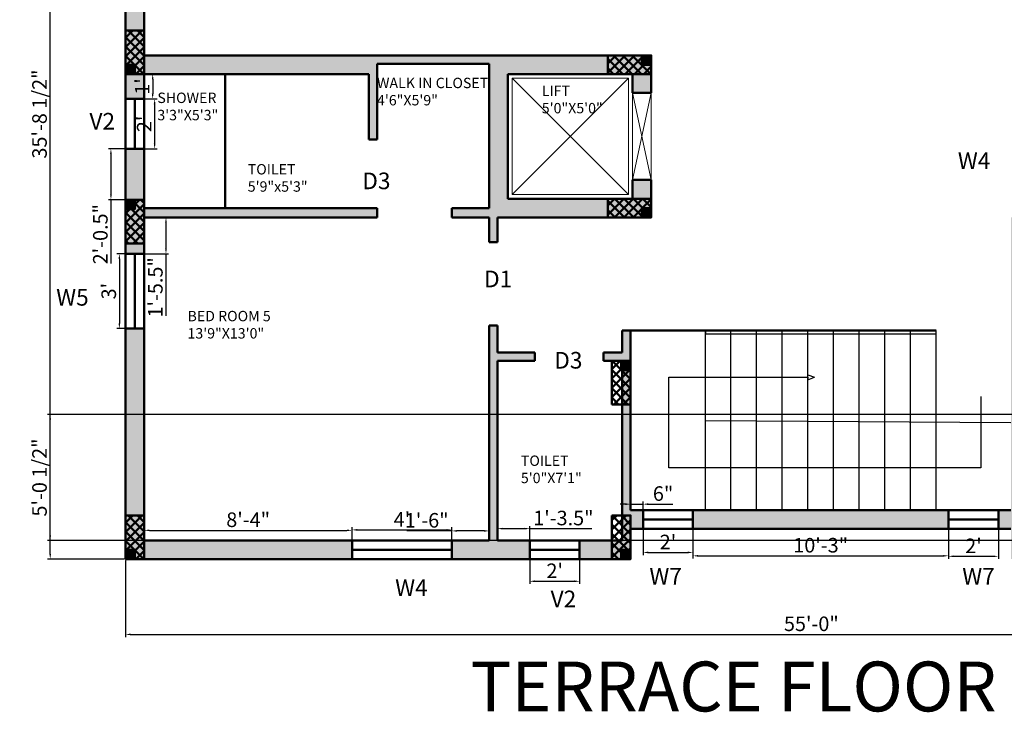
# Model space of a CAD drawing. Units: inches. Extents: x 1749 to 3550, y 1117 to 2383.
# Tile 10 of 15: x 2680 to 3154, y 1169 to 1503. Entities that reach past the tile are written whole.
import ezdxf

# ---------------------------------------------------------------- set-up
doc = ezdxf.new("R2010")
doc.units = ezdxf.units.IN
for name, color, linetype, lineweight in [('A-ANNO-DIMS', 2, 'Continuous', 18), ('A-ANNO-TEXT', 3, 'Continuous', 18), ('A-AREA-IDEN', 7, 'Continuous', 18), ('A-COLS', 10, 'Continuous', 50), ('A-EQPM', 8, 'Continuous', 18), ('A-FLOR-STRS', 53, 'Continuous', 25), ('A-WALL', 7, 'Continuous', 50), ('A-WALL-PATT', 8, 'Continuous', 13)]:
    doc.layers.add(name, color=color, linetype=linetype, lineweight=lineweight)
doc.styles.get("Standard").update_dxf_attribs({"font": 'arial.ttf'})
doc.dimstyles.new('ISO-25', dxfattribs={"dimtxt": 7, "dimasz": 2.5, "dimexe": 1.25, "dimexo": 0.625, "dimtad": 1, "dimdec": 1, "dimlunit": 3, "dimtxsty": 'Standard', "dimcen": 2.5, "dimadec": 0, "dimazin": 0, "dimtfac": 1, "dimtdec": 1, "dimtmove": 0, "dimatfit": 3, "dimfxl": 1, "dimarcsym": 0})

# ---------------------------------------------------------------- blocks, each defined once
blk = doc.blocks.new('*D107')
at = {"layer": 'A-ANNO-DIMS', "color": 0, "lineweight": -2, "ltscale": 0.5, "transparency": 16777216}
for p, q in [((2740.46, 1476.39), (2745.15, 1476.39)), ((2743.9, 1473.89), (2743.9, 1466.89)), ((2740.46, 1464.39), (2745.15, 1464.39))]:
    blk.add_line(p, q, dxfattribs=at)
at = {"layer": 'A-ANNO-DIMS', "color": 0, "ltscale": 0.5, "transparency": 16777216}
for points in [[(2743.48, 1473.89), (2744.31, 1473.89), (2743.9, 1476.39)], [(2743.48, 1466.89), (2744.31, 1466.89), (2743.9, 1464.39)]]:
    blk.add_solid(points, dxfattribs=at)
at = {"layer": 'Defpoints', "color": 0, "ltscale": 0.5, "transparency": 16777216}
for p in [(2739.84, 1476.39), (2739.84, 1464.39), (2743.9, 1464.39)]:
    blk.add_point(p, dxfattribs=at)
at = {"layer": 'A-ANNO-DIMS', "color": 0, "ltscale": 0.5, "transparency": 16777216, "insert": (2739.76, 1470.39), "char_height": 7, "attachment_point": 5, "rotation": 90}
blk.add_mtext("1'", dxfattribs=at)
blk = doc.blocks.new('*D108')
at = {"layer": 'A-ANNO-DIMS', "color": 0, "lineweight": -2, "ltscale": 0.5, "transparency": 16777216}
for p, q in [((2740.46, 1464.39), (2746.09, 1464.39)), ((2744.84, 1461.89), (2744.84, 1442.89)), ((2740.46, 1440.39), (2746.09, 1440.39))]:
    blk.add_line(p, q, dxfattribs=at)
at = {"layer": 'A-ANNO-DIMS', "color": 0, "ltscale": 0.5, "transparency": 16777216}
for points in [[(2744.42, 1461.89), (2745.25, 1461.89), (2744.84, 1464.39)], [(2744.42, 1442.89), (2745.25, 1442.89), (2744.84, 1440.39)]]:
    blk.add_solid(points, dxfattribs=at)
at = {"layer": 'Defpoints', "color": 0, "ltscale": 0.5, "transparency": 16777216}
for p in [(2739.84, 1464.39), (2739.84, 1440.39), (2744.84, 1440.39)]:
    blk.add_point(p, dxfattribs=at)
at = {"layer": 'A-ANNO-DIMS', "color": 0, "ltscale": 0.5, "transparency": 16777216, "insert": (2740.7, 1452.39), "char_height": 7, "attachment_point": 5, "rotation": 90}
blk.add_mtext("2'", dxfattribs=at)
blk = doc.blocks.new('*D109')
at = {"layer": 'A-ANNO-DIMS', "color": 0, "lineweight": -2, "ltscale": 0.5, "transparency": 16777216}
for p, q in [((2730.21, 1440.39), (2722.56, 1440.39)), ((2723.81, 1437.89), (2723.81, 1418.37)), ((2730.21, 1415.87), (2722.56, 1415.87)), ((2723.81, 1415.87), (2723.81, 1385.23))]:
    blk.add_line(p, q, dxfattribs=at)
at = {"layer": 'A-ANNO-DIMS', "color": 0, "ltscale": 0.5, "transparency": 16777216}
for points in [[(2723.39, 1437.89), (2724.22, 1437.89), (2723.81, 1440.39)], [(2723.39, 1418.37), (2724.22, 1418.37), (2723.81, 1415.87)]]:
    blk.add_solid(points, dxfattribs=at)
at = {"layer": 'Defpoints', "color": 0, "ltscale": 0.5, "transparency": 16777216}
for p in [(2730.84, 1440.39), (2723.81, 1415.87), (2730.84, 1415.87)]:
    blk.add_point(p, dxfattribs=at)
at = {"layer": 'A-ANNO-DIMS', "color": 0, "ltscale": 0.5, "transparency": 16777216, "insert": (2719.61, 1399.3), "char_height": 7, "attachment_point": 5, "rotation": 90}
blk.add_mtext('2\'-0.5"', dxfattribs=at)
blk = doc.blocks.new('*D110')
at = {"layer": 'A-ANNO-DIMS', "color": 0, "lineweight": -2, "ltscale": 0.5, "transparency": 16777216}
for p, q in [((2740.46, 1407.39), (2751.54, 1407.39)), ((2750.29, 1404.89), (2750.29, 1392.39)), ((2740.46, 1389.89), (2751.54, 1389.89)), ((2750.29, 1389.89), (2750.29, 1360.03))]:
    blk.add_line(p, q, dxfattribs=at)
at = {"layer": 'A-ANNO-DIMS', "color": 0, "ltscale": 0.5, "transparency": 16777216}
for points in [[(2749.87, 1404.89), (2750.71, 1404.89), (2750.29, 1407.39)], [(2749.87, 1392.39), (2750.71, 1392.39), (2750.29, 1389.89)]]:
    blk.add_solid(points, dxfattribs=at)
at = {"layer": 'Defpoints', "color": 0, "ltscale": 0.5, "transparency": 16777216}
for p in [(2739.84, 1407.39), (2739.84, 1389.89), (2750.29, 1389.89)]:
    blk.add_point(p, dxfattribs=at)
at = {"layer": 'A-ANNO-DIMS', "color": 0, "ltscale": 0.5, "transparency": 16777216, "insert": (2746.09, 1373.71), "char_height": 7, "attachment_point": 5, "rotation": 90}
blk.add_mtext('1\'-5.5"', dxfattribs=at)
blk = doc.blocks.new('*D111')
at = {"layer": 'A-ANNO-DIMS', "color": 0, "lineweight": -2, "ltscale": 0.5, "transparency": 16777216}
for p, q in [((2730.21, 1389.89), (2726.61, 1389.89)), ((2727.86, 1387.39), (2727.86, 1356.39)), ((2730.21, 1353.89), (2726.61, 1353.89))]:
    blk.add_line(p, q, dxfattribs=at)
at = {"layer": 'A-ANNO-DIMS', "color": 0, "ltscale": 0.5, "transparency": 16777216}
for points in [[(2727.45, 1387.39), (2728.28, 1387.39), (2727.86, 1389.89)], [(2727.45, 1356.39), (2728.28, 1356.39), (2727.86, 1353.89)]]:
    blk.add_solid(points, dxfattribs=at)
at = {"layer": 'Defpoints', "color": 0, "ltscale": 0.5, "transparency": 16777216}
for p in [(2730.84, 1389.89), (2727.86, 1353.89), (2730.84, 1353.89)]:
    blk.add_point(p, dxfattribs=at)
at = {"layer": 'A-ANNO-DIMS', "color": 0, "ltscale": 0.5, "transparency": 16777216, "insert": (2723.66, 1371.89), "char_height": 7, "attachment_point": 5, "rotation": 90}
blk.add_mtext("3'", dxfattribs=at)
blk = doc.blocks.new('*D112')
at = {"layer": 'A-ANNO-DIMS', "color": 0, "lineweight": -2, "ltscale": 0.5, "transparency": 16777216}
for p, q in [((2739.84, 1252.51), (2739.84, 1257.99)), ((2742.34, 1256.74), (2837.34, 1256.74)), ((2839.84, 1252.51), (2839.84, 1257.99))]:
    blk.add_line(p, q, dxfattribs=at)
at = {"layer": 'A-ANNO-DIMS', "color": 0, "ltscale": 0.5, "transparency": 16777216}
for points in [[(2742.34, 1257.15), (2742.34, 1256.32), (2739.84, 1256.74)], [(2837.34, 1257.15), (2837.34, 1256.32), (2839.84, 1256.74)]]:
    blk.add_solid(points, dxfattribs=at)
at = {"layer": 'Defpoints', "color": 0, "ltscale": 0.5, "transparency": 16777216}
for p in [(2839.84, 1256.74), (2739.84, 1251.89), (2839.84, 1251.89)]:
    blk.add_point(p, dxfattribs=at)
at = {"layer": 'A-ANNO-DIMS', "color": 0, "ltscale": 0.5, "transparency": 16777216, "insert": (2789.84, 1260.93), "char_height": 7, "attachment_point": 5}
blk.add_mtext('8\'-4"', dxfattribs=at)
blk = doc.blocks.new('*D113')
at = {"layer": 'A-ANNO-DIMS', "color": 0, "lineweight": -2, "ltscale": 0.5, "transparency": 16777216}
for p, q in [((2839.84, 1252.51), (2839.84, 1258.21)), ((2842.34, 1256.96), (2885.34, 1256.96)), ((2887.84, 1252.51), (2887.84, 1258.21))]:
    blk.add_line(p, q, dxfattribs=at)
at = {"layer": 'A-ANNO-DIMS', "color": 0, "ltscale": 0.5, "transparency": 16777216}
for points in [[(2842.34, 1257.37), (2842.34, 1256.54), (2839.84, 1256.96)], [(2885.34, 1257.37), (2885.34, 1256.54), (2887.84, 1256.96)]]:
    blk.add_solid(points, dxfattribs=at)
at = {"layer": 'Defpoints', "color": 0, "ltscale": 0.5, "transparency": 16777216}
for p in [(2887.84, 1256.96), (2839.84, 1251.89), (2887.84, 1251.89)]:
    blk.add_point(p, dxfattribs=at)
at = {"layer": 'A-ANNO-DIMS', "color": 0, "ltscale": 0.5, "transparency": 16777216, "insert": (2863.84, 1261.08), "char_height": 7, "attachment_point": 5}
blk.add_mtext("4'", dxfattribs=at)
blk = doc.blocks.new('*D114')
at = {"layer": 'A-ANNO-DIMS', "color": 0, "lineweight": -2, "ltscale": 0.5, "transparency": 16777216}
for p, q in [((2887.84, 1256.46), (2866.14, 1256.46)), ((2887.84, 1252.51), (2887.84, 1257.71)), ((2903.34, 1256.46), (2890.34, 1256.46)), ((2905.84, 1252.51), (2905.84, 1257.71))]:
    blk.add_line(p, q, dxfattribs=at)
at = {"layer": 'A-ANNO-DIMS', "color": 0, "ltscale": 0.5, "transparency": 16777216}
for points in [[(2890.34, 1256.88), (2890.34, 1256.05), (2887.84, 1256.46)], [(2903.34, 1256.88), (2903.34, 1256.05), (2905.84, 1256.46)]]:
    blk.add_solid(points, dxfattribs=at)
at = {"layer": 'Defpoints', "color": 0, "ltscale": 0.5, "transparency": 16777216}
for p in [(2887.84, 1256.46), (2887.84, 1251.89), (2905.84, 1251.89)]:
    blk.add_point(p, dxfattribs=at)
at = {"layer": 'A-ANNO-DIMS', "color": 0, "ltscale": 0.5, "transparency": 16777216, "insert": (2875.74, 1260.66), "char_height": 7, "attachment_point": 5}
blk.add_mtext('1\'-6"', dxfattribs=at)
blk = doc.blocks.new('*D115')
at = {"layer": 'A-ANNO-DIMS', "color": 0, "lineweight": -2, "ltscale": 0.5, "transparency": 16777216}
for p, q in [((2909.84, 1252.51), (2909.84, 1258.81)), ((2912.34, 1257.56), (2922.84, 1257.56)), ((2925.34, 1252.51), (2925.34, 1258.81)), ((2925.34, 1257.56), (2955.19, 1257.56))]:
    blk.add_line(p, q, dxfattribs=at)
at = {"layer": 'A-ANNO-DIMS', "color": 0, "ltscale": 0.5, "transparency": 16777216}
for points in [[(2912.34, 1257.98), (2912.34, 1257.14), (2909.84, 1257.56)], [(2922.84, 1257.98), (2922.84, 1257.14), (2925.34, 1257.56)]]:
    blk.add_solid(points, dxfattribs=at)
at = {"layer": 'Defpoints', "color": 0, "ltscale": 0.5, "transparency": 16777216}
for p in [(2925.34, 1257.56), (2909.84, 1251.89), (2925.34, 1251.89)]:
    blk.add_point(p, dxfattribs=at)
at = {"layer": 'A-ANNO-DIMS', "color": 0, "ltscale": 0.5, "transparency": 16777216, "insert": (2941.51, 1261.76), "char_height": 7, "attachment_point": 5}
blk.add_mtext('1\'-3.5"', dxfattribs=at)
blk = doc.blocks.new('*D116')
at = {"layer": 'A-ANNO-DIMS', "color": 0, "lineweight": -2, "ltscale": 0.5, "transparency": 16777216}
for p, q in [((2925.34, 1242.26), (2925.34, 1230.97)), ((2949.34, 1242.26), (2949.34, 1230.97)), ((2927.84, 1232.22), (2946.84, 1232.22))]:
    blk.add_line(p, q, dxfattribs=at)
at = {"layer": 'A-ANNO-DIMS', "color": 0, "ltscale": 0.5, "transparency": 16777216}
for points in [[(2927.84, 1232.63), (2927.84, 1231.8), (2925.34, 1232.22)], [(2946.84, 1232.63), (2946.84, 1231.8), (2949.34, 1232.22)]]:
    blk.add_solid(points, dxfattribs=at)
at = {"layer": 'Defpoints', "color": 0, "ltscale": 0.5, "transparency": 16777216}
for p in [(2925.34, 1242.89), (2949.34, 1242.89), (2949.34, 1232.22)]:
    blk.add_point(p, dxfattribs=at)
at = {"layer": 'A-ANNO-DIMS', "color": 0, "ltscale": 0.5, "transparency": 16777216, "insert": (2937.34, 1236.36), "char_height": 7, "attachment_point": 5}
blk.add_mtext("2'", dxfattribs=at)
blk = doc.blocks.new('*D117')
at = {"layer": 'A-ANNO-DIMS', "color": 0, "lineweight": -2, "ltscale": 0.5, "transparency": 16777216}
for p, q in [((2973.84, 1267.01), (2973.84, 1270.59)), ((2979.84, 1267.01), (2979.84, 1270.59)), ((2971.34, 1269.34), (2968.84, 1269.34)), ((2973.84, 1269.34), (2979.84, 1269.34)), ((2982.34, 1269.34), (2994.17, 1269.34))]:
    blk.add_line(p, q, dxfattribs=at)
at = {"layer": 'A-ANNO-DIMS', "color": 0, "ltscale": 0.5, "transparency": 16777216}
for points in [[(2971.34, 1269.76), (2971.34, 1268.92), (2973.84, 1269.34)], [(2982.34, 1269.76), (2982.34, 1268.92), (2979.84, 1269.34)]]:
    blk.add_solid(points, dxfattribs=at)
at = {"layer": 'Defpoints', "color": 0, "ltscale": 0.5, "transparency": 16777216}
for p in [(2973.84, 1266.39), (2979.84, 1269.34), (2979.84, 1266.39)]:
    blk.add_point(p, dxfattribs=at)
at = {"layer": 'A-ANNO-DIMS', "color": 0, "ltscale": 0.5, "transparency": 16777216, "insert": (2989.5, 1273.54), "char_height": 7, "attachment_point": 5}
blk.add_mtext('6"', dxfattribs=at)
blk = doc.blocks.new('*D118')
at = {"layer": 'A-ANNO-DIMS', "color": 0, "lineweight": -2, "ltscale": 0.5, "transparency": 16777216}
for p, q in [((2979.84, 1256.76), (2979.84, 1244.85)), ((3003.84, 1256.76), (3003.84, 1244.85)), ((2982.34, 1246.1), (3001.34, 1246.1))]:
    blk.add_line(p, q, dxfattribs=at)
at = {"layer": 'A-ANNO-DIMS', "color": 0, "ltscale": 0.5, "transparency": 16777216}
for points in [[(2982.34, 1246.51), (2982.34, 1245.68), (2979.84, 1246.1)], [(3001.34, 1246.51), (3001.34, 1245.68), (3003.84, 1246.1)]]:
    blk.add_solid(points, dxfattribs=at)
at = {"layer": 'Defpoints', "color": 0, "ltscale": 0.5, "transparency": 16777216}
for p in [(2979.84, 1257.39), (3003.84, 1257.39), (3003.84, 1246.1)]:
    blk.add_point(p, dxfattribs=at)
at = {"layer": 'A-ANNO-DIMS', "color": 0, "ltscale": 0.5, "transparency": 16777216, "insert": (2991.84, 1250.23), "char_height": 7, "attachment_point": 5}
blk.add_mtext("2'", dxfattribs=at)
blk = doc.blocks.new('*D119')
at = {"layer": 'A-ANNO-DIMS', "color": 0, "lineweight": -2, "ltscale": 0.5, "transparency": 16777216}
for p, q in [((3003.84, 1256.76), (3003.84, 1243.22)), ((3126.84, 1256.76), (3126.84, 1243.22)), ((3006.34, 1244.47), (3124.34, 1244.47))]:
    blk.add_line(p, q, dxfattribs=at)
at = {"layer": 'A-ANNO-DIMS', "color": 0, "ltscale": 0.5, "transparency": 16777216}
for points in [[(3006.34, 1244.88), (3006.34, 1244.05), (3003.84, 1244.47)], [(3124.34, 1244.88), (3124.34, 1244.05), (3126.84, 1244.47)]]:
    blk.add_solid(points, dxfattribs=at)
at = {"layer": 'Defpoints', "color": 0, "ltscale": 0.5, "transparency": 16777216}
for p in [(3003.84, 1257.39), (3126.84, 1257.39), (3126.84, 1244.47)]:
    blk.add_point(p, dxfattribs=at)
at = {"layer": 'A-ANNO-DIMS', "color": 0, "ltscale": 0.5, "transparency": 16777216, "insert": (3065.34, 1248.67), "char_height": 7, "attachment_point": 5}
blk.add_mtext('10\'-3"', dxfattribs=at)
blk = doc.blocks.new('*D120')
at = {"layer": 'A-ANNO-DIMS', "color": 0, "lineweight": -2, "ltscale": 0.5, "transparency": 16777216}
for p, q in [((3126.84, 1256.76), (3126.84, 1242.98)), ((3150.84, 1256.76), (3150.84, 1242.98)), ((3129.34, 1244.23), (3148.34, 1244.23))]:
    blk.add_line(p, q, dxfattribs=at)
at = {"layer": 'A-ANNO-DIMS', "color": 0, "ltscale": 0.5, "transparency": 16777216}
for points in [[(3129.34, 1244.65), (3129.34, 1243.82), (3126.84, 1244.23)], [(3148.34, 1244.65), (3148.34, 1243.82), (3150.84, 1244.23)]]:
    blk.add_solid(points, dxfattribs=at)
at = {"layer": 'Defpoints', "color": 0, "ltscale": 0.5, "transparency": 16777216}
for p in [(3126.84, 1257.39), (3150.84, 1257.39), (3150.84, 1244.23)]:
    blk.add_point(p, dxfattribs=at)
at = {"layer": 'A-ANNO-DIMS', "color": 0, "ltscale": 0.5, "transparency": 16777216, "insert": (3138.84, 1248.37), "char_height": 7, "attachment_point": 5}
blk.add_mtext("2'", dxfattribs=at)
blk = doc.blocks.new('LIFT-A')
at = {"ltscale": 0.2}
for p, q in [((0, 56), (56, 56)), ((0, 56), (0, 0)), ((56, 56), (0, 0)), ((0, 56), (56, 0)), ((56, 56), (56, 0)), ((0, 0), (56, 0))]:
    blk.add_line(p, q, dxfattribs=at)
blk = doc.blocks.new('*D199')
at = {"layer": 'A-ANNO-DIMS', "color": 0, "lineweight": -2, "ltscale": 0.5, "transparency": 16777216}
for p, q in [((2730.84, 1242.26), (2730.84, 1205.39)), ((3390.84, 1242.26), (3390.84, 1205.39)), ((2733.34, 1206.64), (3388.34, 1206.64))]:
    blk.add_line(p, q, dxfattribs=at)
at = {"layer": 'A-ANNO-DIMS', "color": 0, "ltscale": 0.5, "transparency": 16777216}
for points in [[(2733.34, 1207.05), (2733.34, 1206.22), (2730.84, 1206.64)], [(3388.34, 1207.05), (3388.34, 1206.22), (3390.84, 1206.64)]]:
    blk.add_solid(points, dxfattribs=at)
at = {"layer": 'Defpoints', "color": 0, "ltscale": 0.5, "transparency": 16777216}
for p in [(2730.84, 1242.89), (3390.84, 1242.89), (3390.84, 1206.64)]:
    blk.add_point(p, dxfattribs=at)
at = {"layer": 'A-ANNO-DIMS', "color": 0, "ltscale": 0.5, "transparency": 16777216, "insert": (3060.84, 1210.84), "char_height": 7, "attachment_point": 5}
blk.add_mtext('55\'-0"', dxfattribs=at)
blk = doc.blocks.new('*D200')
at = {"layer": 'A-ANNO-DIMS', "color": 0, "lineweight": -2, "ltscale": 0.5, "transparency": 16777216}
for p, q in [((2730.21, 1671.39), (2693.34, 1671.39)), ((2694.59, 1245.39), (2694.59, 1668.89)), ((2730.21, 1242.89), (2693.34, 1242.89))]:
    blk.add_line(p, q, dxfattribs=at)
at = {"layer": 'A-ANNO-DIMS', "color": 0, "ltscale": 0.5, "transparency": 16777216}
for points in [[(2694.17, 1668.89), (2695, 1668.89), (2694.59, 1671.39)], [(2694.17, 1245.39), (2695, 1245.39), (2694.59, 1242.89)]]:
    blk.add_solid(points, dxfattribs=at)
at = {"layer": 'Defpoints', "color": 0, "ltscale": 0.5, "transparency": 16777216}
for p in [(2694.59, 1671.39), (2730.84, 1671.39), (2730.84, 1242.89)]:
    blk.add_point(p, dxfattribs=at)
at = {"layer": 'A-ANNO-DIMS', "color": 0, "ltscale": 0.5, "transparency": 16777216, "insert": (2690.34, 1457.14), "char_height": 7, "attachment_point": 5, "rotation": 90}
blk.add_mtext('35\'-8 1/2"', dxfattribs=at)
blk = doc.blocks.new('*D204')
at = {"layer": 'A-ANNO-DIMS', "color": 0, "lineweight": -2, "ltscale": 0.5, "transparency": 16777216}
for p, q in [((3202.94, 1312.45), (2693.34, 1312.45)), ((2694.59, 1254.39), (2694.59, 1309.95)), ((3165.21, 1251.89), (2693.34, 1251.89))]:
    blk.add_line(p, q, dxfattribs=at)
at = {"layer": 'A-ANNO-DIMS', "color": 0, "ltscale": 0.5, "transparency": 16777216}
for points in [[(2694.17, 1309.95), (2695, 1309.95), (2694.59, 1312.45)], [(2694.17, 1254.39), (2695, 1254.39), (2694.59, 1251.89)]]:
    blk.add_solid(points, dxfattribs=at)
at = {"layer": 'Defpoints', "color": 0, "ltscale": 0.5, "transparency": 16777216}
for p in [(2694.59, 1312.45), (3203.57, 1312.45), (3165.84, 1251.89)]:
    blk.add_point(p, dxfattribs=at)
at = {"layer": 'A-ANNO-DIMS', "color": 0, "ltscale": 0.5, "transparency": 16777216, "insert": (2690.34, 1282.17), "char_height": 7, "attachment_point": 5, "rotation": 90}
blk.add_mtext('5\'-0 1/2"', dxfattribs=at)

msp = doc.modelspace()

# ---------------------------------------------------------------- hatches: boundary and pattern name
at = {"layer": 'A-COLS', "ltscale": 10}
h = msp.add_hatch(dxfattribs=at)
h.set_pattern_fill('ANSI37', color=256, angle=270)
h.set_pattern_definition([(315, (1372.7294, 3148.631), (2.245064, 2.245064), []), (45, (1372.7294, 3148.631), (-2.245064, 2.245064), [])])
h.paths.add_polyline_path([(2730.84, 1476.39), (2739.84, 1476.39), (2739.84, 1497.39), (2730.84, 1497.39)])
h = msp.add_hatch(dxfattribs=at)
h.set_pattern_fill('ANSI37', color=256, angle=360)
h.set_pattern_definition([(45, (1311.591, 90.5872), (-2.245064, 2.245064), []), (135, (1311.591, 90.5872), (-2.245064, -2.245064), [])])
h.paths.add_polyline_path([(2962.84, 1485.39), (2962.84, 1476.39), (2983.84, 1476.39), (2983.84, 1485.39)])
h = msp.add_hatch(color=256, dxfattribs=at)
h.dxf.hatch_style = 1
h.paths.add_polyline_path([(2983.84, 1485.39), (2979.34, 1485.39), (2979.34, 1480.89), (2983.84, 1480.89)])
h = msp.add_hatch(color=256, dxfattribs=at)
h.dxf.hatch_style = 1
h.paths.add_polyline_path([(2735.34, 1476.39), (2735.34, 1480.89), (2730.84, 1480.89), (2730.84, 1476.39)])
h = msp.add_hatch(color=256, dxfattribs=at)
h.dxf.hatch_style = 1
h.paths.add_polyline_path([(2730.84, 1415.87), (2730.84, 1411.37), (2735.34, 1411.37), (2735.34, 1415.87)])
h = msp.add_hatch(dxfattribs=at)
h.set_pattern_fill('ANSI37', color=256, angle=90)
h.set_pattern_definition([(135, (4078.1257, -256.377), (-2.245064, -2.245064), []), (225, (4078.1257, -256.377), (2.245064, -2.245064), [])])
h.paths.add_polyline_path([(2730.84, 1394.87), (2739.84, 1394.87), (2739.84, 1415.87), (2730.84, 1415.87)])
h = msp.add_hatch(dxfattribs=at)
h.set_pattern_fill('ANSI37', color=256, angle=360)
h.set_pattern_definition([(45, (1311.591, 49.2816), (-2.245064, 2.245064), []), (135, (1311.591, 49.2816), (-2.245064, -2.245064), [])])
h.paths.add_polyline_path([(2983.84, 1407.39), (2983.84, 1416.39), (2962.84, 1416.39), (2962.84, 1407.39)])
h = msp.add_hatch(color=256, dxfattribs=at)
h.dxf.hatch_style = 1
h.paths.add_polyline_path([(2983.84, 1411.89), (2979.34, 1411.89), (2979.34, 1407.39), (2983.84, 1407.39)])
h = msp.add_hatch(dxfattribs=at)
h.set_pattern_fill('ANSI37', color=256, angle=90)
h.set_pattern_definition([(135, (4331.9415, -333.8625), (-2.245064, -2.245064), []), (225, (4331.9415, -333.8625), (2.245064, -2.245064), [])])
h.paths.add_polyline_path([(2973.84, 1338.38), (2964.84, 1338.38), (2964.84, 1317.38), (2973.84, 1317.38)])
h = msp.add_hatch(color=256, dxfattribs=at)
h.dxf.hatch_style = 1
h.paths.add_polyline_path([(2969.34, 1338.38), (2969.34, 1333.88), (2973.84, 1333.88), (2973.84, 1338.38)])
h = msp.add_hatch(dxfattribs=at)
h.set_pattern_fill('ANSI37', color=256, angle=270)
h.set_pattern_definition([(315, (1372.7294, 2915.132), (2.245064, 2.245064), []), (45, (1372.7294, 2915.132), (-2.245064, 2.245064), [])])
h.paths.add_polyline_path([(2730.84, 1242.89), (2739.84, 1242.89), (2739.84, 1263.89), (2730.84, 1263.89)])
h = msp.add_hatch(dxfattribs=at)
h.set_pattern_fill('ANSI37', color=256, angle=270)
h.set_pattern_definition([(315, (1583.087, 2915.132), (2.245064, 2.245064), []), (45, (1583.087, 2915.132), (-2.245064, 2.245064), [])])
h.paths.add_polyline_path([(2973.84, 1263.89), (2964.84, 1263.89), (2964.84, 1242.89), (2973.84, 1242.89)])
h = msp.add_hatch(color=256, dxfattribs=at)
h.dxf.hatch_style = 1
h.paths.add_polyline_path([(2735.34, 1242.89), (2735.34, 1247.39), (2730.84, 1247.39), (2730.84, 1242.89)])
h = msp.add_hatch(color=256, dxfattribs=at)
h.dxf.hatch_style = 1
h.paths.add_polyline_path([(2973.84, 1242.89), (2973.84, 1247.39), (2969.34, 1247.39), (2969.34, 1242.89)])
at = {"layer": 'A-WALL-PATT', "ltscale": 0.5}
h = msp.add_hatch(color=256, dxfattribs=at)
h.dxf.hatch_style = 1
h.paths.add_polyline_path([(2798.34, 1662.39), (2798.34, 1671.39), (2730.84, 1671.39), (2730.84, 1464.39), (2739.84, 1464.39), (2739.84, 1476.39), (2847.84, 1476.39), (2847.84, 1444.89), (2851.84, 1444.89), (2851.84, 1481.39), (2905.84, 1481.39), (2905.84, 1411.89), (2887.84, 1411.89), (2887.84, 1407.39), (2905.84, 1407.39), (2905.84, 1395.39), (2909.84, 1395.39), (2909.84, 1407.39), (2973.84, 1407.39), (2983.84, 1407.39), (2983.84, 1425.39), (2974.84, 1425.39), (2974.84, 1416.39), (2914.84, 1416.39), (2914.84, 1476.39), (2974.84, 1476.39), (2974.84, 1467.39), (2983.84, 1467.39), (2983.84, 1476.39), (2983.84, 1485.39), (2739.84, 1485.39), (2739.84, 1662.39)])
h = msp.add_hatch(color=256, dxfattribs=at)
h.dxf.hatch_style = 1
h.paths.add_polyline_path([(2739.84, 1407.39), (2851.84, 1407.39), (2851.84, 1411.89), (2847.84, 1411.89), (2739.84, 1411.89), (2739.84, 1440.39), (2730.84, 1440.39), (2730.84, 1389.89), (2739.84, 1389.89)])
h = msp.add_hatch(color=256, dxfattribs=at)
h.dxf.hatch_style = 1
h.paths.add_polyline_path([(3156.84, 1266.39), (3150.84, 1266.39), (3150.84, 1257.39), (3156.84, 1257.39), (3156.84, 1242.89), (3165.84, 1242.89), (3165.84, 1251.89), (3165.84, 1407.39), (3156.84, 1407.39)])
h = msp.add_hatch(color=256, dxfattribs=at)
h.dxf.hatch_style = 1
h.paths.add_polyline_path([(2905.84, 1251.89), (2887.84, 1251.89), (2887.84, 1242.89), (2925.34, 1242.89), (2925.34, 1251.89), (2909.84, 1251.89), (2909.84, 1338.39), (2927.84, 1338.39), (2927.84, 1342.39), (2909.84, 1342.39), (2909.84, 1355.39), (2905.84, 1355.39)])
h = msp.add_hatch(color=256, dxfattribs=at)
h.dxf.hatch_style = 1
h.paths.add_polyline_path([(2739.84, 1353.89), (2730.84, 1353.89), (2730.84, 1242.89), (2839.84, 1242.89), (2839.84, 1251.89), (2739.84, 1251.89)])
h = msp.add_hatch(color=256, dxfattribs=at)
h.dxf.hatch_style = 1
h.paths.add_polyline_path([(2973.84, 1242.89), (2973.84, 1257.39), (2979.84, 1257.39), (2979.84, 1266.39), (2973.84, 1266.39), (2973.84, 1352.89), (2969.84, 1352.89), (2969.84, 1342.39), (2960.84, 1342.39), (2960.84, 1338.39), (2969.84, 1338.39), (2969.84, 1251.89), (2949.34, 1251.89), (2949.34, 1242.89)])
h = msp.add_hatch(color=256, dxfattribs=at)
h.dxf.hatch_style = 1
h.paths.add_polyline_path([(3126.84, 1257.39), (3126.84, 1266.39), (3003.84, 1266.39), (3003.84, 1257.39)])

# ---------------------------------------------------------------- linework, layer by layer
at = {"layer": 'A-COLS', "ltscale": 10}
for points in [[(2739.84, 1497.39), (2739.84, 1476.39), (2730.84, 1476.39), (2730.84, 1497.39)], [(2962.84, 1476.39), (2983.84, 1476.39), (2983.84, 1485.39), (2962.84, 1485.39)], [(2983.84, 1480.89), (2983.84, 1485.39), (2979.34, 1485.39), (2979.34, 1480.89)], [(2735.34, 1476.39), (2730.84, 1476.39), (2730.84, 1480.89), (2735.34, 1480.89)], [(2735.34, 1415.87), (2730.84, 1415.87), (2730.84, 1411.37), (2735.34, 1411.37)], [(2739.84, 1394.87), (2739.84, 1415.87), (2730.84, 1415.87), (2730.84, 1394.87)], [(2962.84, 1416.39), (2983.84, 1416.39), (2983.84, 1407.39), (2962.84, 1407.39)], [(2983.84, 1411.89), (2983.84, 1407.39), (2979.34, 1407.39), (2979.34, 1411.89)], [(2964.84, 1317.38), (2964.84, 1338.38), (2973.84, 1338.38), (2973.84, 1317.38)], [(2969.34, 1338.38), (2973.84, 1338.38), (2973.84, 1333.88), (2969.34, 1333.88)], [(2739.84, 1263.89), (2739.84, 1242.89), (2730.84, 1242.89), (2730.84, 1263.89)], [(2964.84, 1263.89), (2964.84, 1242.89), (2973.84, 1242.89), (2973.84, 1263.89)], [(2735.34, 1242.89), (2730.84, 1242.89), (2730.84, 1247.39), (2735.34, 1247.39)], [(2969.34, 1242.89), (2973.84, 1242.89), (2973.84, 1247.39), (2969.34, 1247.39)]]:
    msp.add_lwpolyline(points, close=True, dxfattribs=at)
at = {"layer": 'A-EQPM', "ltscale": 0.5}
for p, q in [((2914.84, 1476.39), (2914.84, 1474.39)), ((2974.84, 1467.39), (2974.84, 1425.39)), ((2983.84, 1467.39), (2974.84, 1467.39)), ((2974.84, 1467.39), (2983.84, 1425.39)), ((2974.84, 1425.39), (2983.84, 1467.39)), ((2983.84, 1425.39), (2983.84, 1467.39)), ((2974.84, 1425.39), (2983.84, 1425.39)), ((2983.84, 1425.39), (2974.84, 1425.39))]:
    msp.add_line(p, q, dxfattribs=at)
at = {"layer": 'A-FLOR-STRS', "ltscale": 0.5}
for p, q in [((3009.84, 1266.39), (3009.84, 1352.89)), ((3009.84, 1352.89), (3009.84, 1351.39)), ((3009.84, 1351.39), (3120.84, 1351.39)), ((3022.17, 1266.39), (3022.17, 1352.89)), ((3034.5, 1266.39), (3034.5, 1352.89)), ((3046.84, 1266.39), (3046.84, 1352.89)), ((3059.17, 1266.39), (3059.17, 1352.89)), ((3071.5, 1266.39), (3071.5, 1352.89)), ((3083.84, 1266.39), (3083.84, 1352.89)), ((3096.17, 1266.39), (3096.17, 1352.89)), ((3108.5, 1266.39), (3108.5, 1352.89)), ((3120.84, 1266.39), (3120.84, 1352.89)), ((3120.84, 1266.39), (3120.84, 1351.39)), ((3059.17, 1330.41), (3059.17, 1331.66)), ((3059.17, 1331.66), (3062.37, 1330.41)), ((2992.28, 1286.82), (2992.28, 1330.41)), ((2992.28, 1330.41), (3059.17, 1330.41)), ((3059.17, 1330.41), (3059.17, 1329.16)), ((3059.17, 1329.16), (3062.37, 1330.41)), ((3142.39, 1321.15), (3142.39, 1286.82)), ((3009.84, 1309.64), (3156.84, 1308.64)), ((3142.39, 1286.82), (2992.28, 1286.82))]:
    msp.add_line(p, q, dxfattribs=at)
at = {"layer": 'A-WALL', "ltscale": 0.5}
for p, q in [((2730.84, 1671.39), (2730.84, 1242.89)), ((2739.84, 1662.39), (2739.84, 1485.39)), ((2739.84, 1485.39), (2983.84, 1485.39)), ((2983.84, 1476.39), (2983.84, 1485.39)), ((2851.84, 1481.39), (2851.84, 1444.89)), ((2851.84, 1481.39), (2905.84, 1481.39)), ((2905.84, 1481.39), (2905.84, 1411.89)), ((2739.84, 1476.39), (2847.84, 1476.39)), ((2739.84, 1476.39), (2739.84, 1411.89)), ((2778.84, 1476.39), (2778.84, 1411.89)), ((2778.84, 1476.39), (2778.84, 1411.89)), ((2847.84, 1476.39), (2847.84, 1444.89)), ((2914.84, 1476.39), (2914.84, 1416.39)), ((2914.84, 1476.39), (2974.84, 1476.39)), ((2974.84, 1476.39), (2974.84, 1467.39)), ((2983.84, 1476.39), (2983.84, 1467.39)), ((2739.84, 1464.39), (2730.84, 1464.39)), ((2735.34, 1464.39), (2735.34, 1440.39)), ((2974.84, 1467.39), (2983.84, 1467.39)), ((2739.84, 1440.39), (2730.84, 1440.39)), ((2847.84, 1444.89), (2851.84, 1444.89)), ((2974.84, 1425.39), (2983.84, 1425.39)), ((2974.84, 1425.39), (2974.84, 1416.39)), ((2983.84, 1425.39), (2983.84, 1407.39)), ((2914.84, 1416.39), (2974.84, 1416.39)), ((2739.84, 1411.89), (2847.84, 1411.89)), ((2739.84, 1407.39), (2739.84, 1251.89)), ((2739.84, 1407.39), (2851.84, 1407.39)), ((2847.84, 1411.89), (2851.84, 1411.89)), ((2851.84, 1411.89), (2851.84, 1407.39)), ((2887.84, 1411.89), (2905.84, 1411.89)), ((2887.84, 1411.89), (2887.84, 1407.39)), ((2887.84, 1407.39), (2905.84, 1407.39)), ((2905.84, 1407.39), (2905.84, 1395.39)), ((2909.84, 1407.39), (2909.84, 1395.39)), ((2909.84, 1407.39), (2973.84, 1407.39)), ((2973.84, 1407.39), (2983.84, 1407.39)), ((2905.84, 1395.39), (2909.84, 1395.39)), ((2739.84, 1389.89), (2730.84, 1389.89)), ((2735.34, 1389.89), (2735.34, 1353.89)), ((2905.84, 1355.39), (2909.84, 1355.39)), ((2905.84, 1355.39), (2905.84, 1251.89)), ((2909.84, 1355.39), (2909.84, 1342.39)), ((2739.84, 1353.89), (2730.84, 1353.89)), ((2969.84, 1352.89), (2969.84, 1342.39)), ((2969.84, 1352.89), (2973.84, 1352.89)), ((2973.84, 1352.89), (2973.84, 1266.39)), ((2973.84, 1352.89), (3120.84, 1352.89)), ((2909.84, 1342.39), (2927.84, 1342.39)), ((2927.84, 1342.39), (2927.84, 1338.39)), ((2960.84, 1342.39), (2960.84, 1338.39)), ((2960.84, 1342.39), (2969.84, 1342.39)), ((2909.84, 1338.39), (2927.84, 1338.39)), ((2909.84, 1338.39), (2909.84, 1251.89)), ((2960.84, 1338.39), (2969.84, 1338.39)), ((2969.84, 1338.39), (2969.84, 1251.89)), ((2973.84, 1266.39), (3156.84, 1266.39)), ((2979.84, 1257.39), (2979.84, 1266.39)), ((3003.84, 1257.39), (3003.84, 1266.39)), ((3126.84, 1257.39), (3126.84, 1266.39)), ((3150.84, 1257.39), (3150.84, 1266.39)), ((2979.84, 1261.89), (3003.84, 1261.89)), ((3126.84, 1261.89), (3150.84, 1261.89)), ((2973.84, 1257.39), (3156.84, 1257.39)), ((2973.84, 1257.39), (2973.84, 1242.89)), ((2739.84, 1251.89), (2905.84, 1251.89)), ((2839.84, 1251.89), (2839.84, 1242.89)), ((2887.84, 1251.89), (2887.84, 1242.89)), ((2909.84, 1251.89), (2969.84, 1251.89)), ((2925.34, 1251.89), (2925.34, 1242.89)), ((2949.34, 1251.89), (2949.34, 1242.89)), ((2839.84, 1247.39), (2887.84, 1247.39)), ((2925.34, 1247.39), (2949.34, 1247.39)), ((2730.84, 1242.89), (2973.84, 1242.89))]:
    msp.add_line(p, q, dxfattribs=at)

# ---------------------------------------------------------------- block references
at = {"layer": 'A-EQPM'}
msp.add_blockref('LIFT-A', (2916.84, 1418.39), dxfattribs=at)

# ---------------------------------------------------------------- texts
at = {"layer": 'A-ANNO-TEXT', "ltscale": 0.5}
for s, height, p in [('V2', 8, (2713.45, 1449.67)), ('W4', 8, (3131.33, 1430.67)), ('D3', 8, (2844.76, 1420.97)), ('D1', 8, (2903.35, 1373.75)), ('W5', 8, (2697.47, 1364.9)), ('D3', 8, (2937.13, 1334.61)), ('W7', 8, (2982.91, 1230.62)), ('W7', 8, (3133.46, 1230.62)), ('W4', 8, (2860.58, 1225.13)), ('V2', 8, (2935.37, 1219.71)), ('TERRACE FLOOR', 24, (2896.87, 1169.56))]:
    msp.add_text(s, height=height, dxfattribs=at).set_placement(p)
at = {"layer": 'A-AREA-IDEN', "ltscale": 0.5}
for s, p in [('WALK IN CLOSET', (2851.84, 1469.6)), ('LIFT', (2931.13, 1465.78)), ('SHOWER', (2746.14, 1462.45)), ('4\'6"X5\'9"', (2851.84, 1461.3)), ('3\'3"X5\'3"', (2746.14, 1454.15)), ('5\'0"X5\'0"', (2931.13, 1457.48)), ('TOILET', (2789.64, 1428.05)), ('5\'9"x5\'3"', (2789.64, 1419.75)), ('BED ROOM 5', (2760.66, 1357.38)), ('13\'9"X13\'0"', (2760.66, 1349.08)), ('TOILET', (2921.07, 1287.76)), ('5\'0"X7\'1"', (2921.07, 1279.46))]:
    msp.add_text(s, height=5, dxfattribs=at).set_placement(p)

# ---------------------------------------------------------------- dimensions: what is measured, and where the dimension line sits
at = {"layer": 'A-ANNO-DIMS', "ltscale": 0.5}
for base, p1, p2, override, picture, middle in [((2694.59, 1671.39), (2730.84, 1242.89), (2730.84, 1671.39), {"dimdec": 1, "dimlfac": 1, "dimrnd": 0, "dimzin": 1, "dimdsep": 46, "dimlunit": 4, "dimfrac": 2}, '*D200', (2690.34, 1457.14)), ((2743.9, 1464.39), (2739.84, 1476.39), (2739.84, 1464.39), {"dimclrd": 0, "dimclre": 0, "dimclrt": 0}, '*D107', (2739.76, 1470.39)), ((2744.84, 1440.39), (2739.84, 1464.39), (2739.84, 1440.39), {"dimclrd": 0, "dimclre": 0, "dimclrt": 0}, '*D108', (2740.7, 1452.39)), ((2723.81, 1415.87), (2730.84, 1440.39), (2730.84, 1415.87), {"dimclrd": 0, "dimclre": 0, "dimclrt": 0}, '*D109', (2719.61, 1399.3)), ((2750.29, 1389.89), (2739.84, 1407.39), (2739.84, 1389.89), {"dimclrd": 0, "dimclre": 0, "dimclrt": 0}, '*D110', (2746.09, 1373.71)), ((2727.86, 1353.89), (2730.84, 1389.89), (2730.84, 1353.89), {"dimclrd": 0, "dimclre": 0, "dimclrt": 0}, '*D111', (2723.66, 1371.89)), ((2694.59, 1312.45), (3165.84, 1251.89), (3203.57, 1312.45), {"dimdec": 1, "dimlfac": 1, "dimrnd": 0, "dimzin": 1, "dimdsep": 46, "dimlunit": 4, "dimfrac": 2}, '*D204', (2690.34, 1282.17))]:
    dim = msp.add_linear_dim(base=base, p1=p1, p2=p2, angle=90, dimstyle='ISO-25', override=override, dxfattribs=at)
    dim.commit()
    dim.dimension.update_dxf_attribs({"geometry": picture, "text_midpoint": middle})
for base, p1, p2, override, picture, middle in [((2979.84, 1269.34), (2973.84, 1266.39), (2979.84, 1266.39), {"dimclrd": 0, "dimclre": 0, "dimclrt": 0}, '*D117', (2989.5, 1273.54)), ((2839.84, 1256.74), (2739.84, 1251.89), (2839.84, 1251.89), {"dimclrd": 0, "dimclre": 0, "dimclrt": 0}, '*D112', (2789.84, 1260.93)), ((2887.84, 1256.96), (2839.84, 1251.89), (2887.84, 1251.89), {"dimclrd": 0, "dimclre": 0, "dimclrt": 0}, '*D113', (2863.84, 1261.08)), ((2887.84, 1256.46), (2905.84, 1251.89), (2887.84, 1251.89), {"dimclrd": 0, "dimclre": 0, "dimclrt": 0}, '*D114', (2875.74, 1260.66)), ((2925.34, 1257.56), (2909.84, 1251.89), (2925.34, 1251.89), {"dimclrd": 0, "dimclre": 0, "dimclrt": 0}, '*D115', (2941.51, 1261.76)), ((3003.84, 1246.1), (2979.84, 1257.39), (3003.84, 1257.39), {"dimclrd": 0, "dimclre": 0, "dimclrt": 0}, '*D118', (2991.84, 1250.23)), ((3126.84, 1244.47), (3003.84, 1257.39), (3126.84, 1257.39), {"dimclrd": 0, "dimclre": 0, "dimclrt": 0}, '*D119', (3065.34, 1248.67)), ((3150.84, 1244.23), (3126.84, 1257.39), (3150.84, 1257.39), {"dimclrd": 0, "dimclre": 0, "dimclrt": 0}, '*D120', (3138.84, 1248.37)), ((3390.84, 1206.64), (2730.84, 1242.89), (3390.84, 1242.89), {"dimdec": 1, "dimlfac": 1, "dimrnd": 0, "dimzin": 1, "dimdsep": 46, "dimlunit": 4, "dimfrac": 2}, '*D199', (3060.84, 1210.84)), ((2949.34, 1232.22), (2925.34, 1242.89), (2949.34, 1242.89), {"dimclrd": 0, "dimclre": 0, "dimclrt": 0}, '*D116', (2937.34, 1236.36))]:
    dim = msp.add_linear_dim(base=base, p1=p1, p2=p2, dimstyle='ISO-25', override=override, dxfattribs=at)
    dim.commit()
    dim.dimension.update_dxf_attribs({"geometry": picture, "text_midpoint": middle})

doc.saveas('drawing.dxf')
